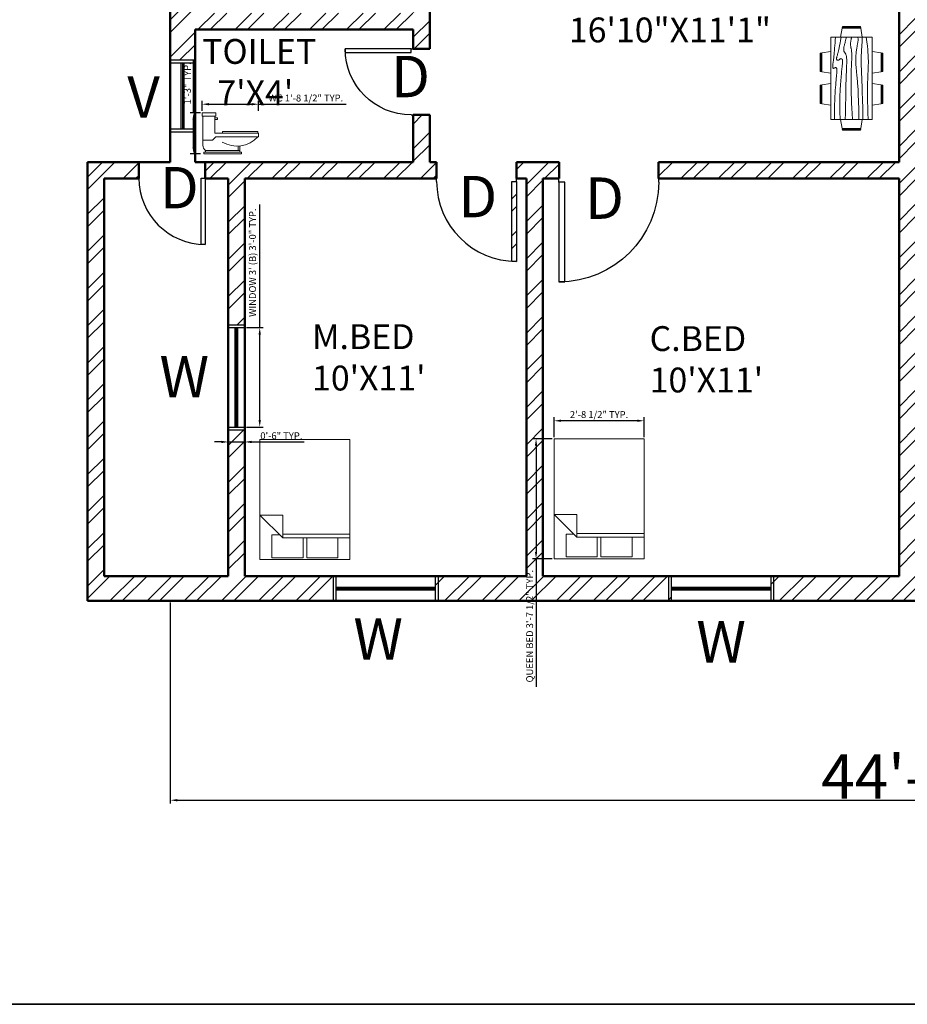
# Model space of a CAD drawing. Units: inches. Extents: x -31842 to -29388, y 18869 to 19743.
# Tile 5 of 12: x -30939 to -30617, y 18869 to 19226. Entities that reach past the tile are written whole.
import ezdxf

# ---------------------------------------------------------------- set-up
doc = ezdxf.new("R2010")
doc.units = ezdxf.units.IN
for name, color, linetype, lineweight in [('A-ANNO-DIMS', 2, 'Continuous', 18), ('A-ANNO-SYMB', 2, 'Continuous', 18), ('A-ANNO-TTLB', 7, 'Continuous', 35), ('A-AREA-IDEN', 3, 'Continuous', 18), ('A-DOOR', 3, 'Continuous', 25), ('A-FLOR-FIXT', 8, 'Continuous', 18), ('A-FURN', 8, 'Continuous', 18), ('A-GLAZ', 4, 'Continuous', 25), ('A-WALL', 7, 'Continuous', 50), ('A-WALL-PATT', 8, 'Continuous', 13)]:
    doc.layers.add(name, color=color, linetype=linetype, lineweight=lineweight)
doc.styles.get("Standard").update_dxf_attribs({"font": 'arial.ttf'})
doc.dimstyles.new('ISO-25', dxfattribs={"dimtxt": 2.5, "dimasz": 2.5, "dimexe": 1.25, "dimexo": 0.625, "dimtad": 1, "dimdec": 0, "dimlunit": 3, "dimtxsty": 'Standard', "dimcen": 2.5, "dimadec": 0, "dimazin": 0, "dimtfac": 1, "dimtdec": 0, "dimtmove": 0, "dimatfit": 3, "dimfxl": 1, "dimarcsym": 0})

# ---------------------------------------------------------------- blocks, each defined once
blk = doc.blocks.new('*U8')
for p, q in [((0, 0), (0, -100)), ((750, 0), (750, -100))]:
    blk.add_line(p, q)
blk.add_lwpolyline([(0, 0), (0, 750), (43.75, 750), (43.75, 0)], close=True)
blk.add_arc((0, 0), 750, 0, 90)
blk = doc.blocks.new('Bed - Queen')
for p, q in [((0, -80.00003), (0, 0)), ((0, 0), (59.99999, 0)), ((59.99999, 0), (59.99999, -80.00003)), ((7.99999, -1.2), (28.79998, -1.2)), ((7.99999, -14.4), (7.99999, -1.2)), ((28.79998, -1.2), (28.79998, -14.4)), ((31.19999, -1.2), (51.99999, -1.2)), ((31.19999, -14.4), (31.19999, -1.2)), ((51.99999, -1.2), (51.99999, -16.4)), ((0, -14.4), (44.8, -14.4)), ((44.8, -16.8), (0, -16.8)), ((59.99999, -29.6), (44.8, -14.4)), ((44.8, -14.4), (44.8, -29.6)), ((51.99999, -16.4), (46.79936, -16.4)), ((44.8, -29.6), (59.99999, -29.6)), ((59.99999, -80.00003), (0, -80.00003))]:
    blk.add_line(p, q)
blk = doc.blocks.new('Toilet - side')
for p, q in [((0.5, 5), (0.5, 22)), ((7.5, 22), (7.5, 12)), ((7.5, 21), (9, 21)), ((9, 20), (7.5, 20)), ((9, 21), (9, 20)), ((7.5, 12), (33, 12)), ((32.5, 13), (12, 13)), ((12, 13), (12, 12)), ((32.5, 12), (32.5, 13)), ((33, 12), (33, 10)), ((6, 8), (0.5, 8)), ((8, 10), (6, 8)), ((33, 10), (8, 10)), ((22, 2), (2, 2)), ((2, 2), (2, 1)), ((21, 4.5), (21, 2)), ((22, 2), (22, 4.54)), ((22, 1), (22, 2))]:
    blk.add_line(p, q)
for points in [[(0, 22), (0, 24), (8, 24), (8, 22)], [(1, 0), (1, 1), (23, 1), (23, 0)]]:
    blk.add_lwpolyline(points, close=True)
for centre, radius, start, end in [((20.3, 20.7), 16.23, 238.18715, 318.77023), ((3.75, 4.75), 3.26, 175.6013, 237.5288)]:
    blk.add_arc(centre, radius, start, end)
blk = doc.blocks.new('Dining Set - 36 x 72 in.')
for p, q in [((-22.2343, 26.00059), (-23.4847, 17.99762)), ((-22.2304, 26), (-5.7608, 26)), ((-22, 27.5), (-22.1562, 26.50042)), ((-5.8416, 26.5), (-22.1534, 26.5)), ((-22, 27.5), (-6, 27.5)), ((-5.8437, 26.49966), (-6, 27.5)), ((-4.5152, 17.99762), (-5.7655, 25.99926)), ((5.7657, 26.00059), (4.5153, 17.99762)), ((5.7696, 26), (22.2392, 26)), ((6, 27.5), (5.8438, 26.50042)), ((22.1584, 26.5), (5.8466, 26.5)), ((6, 27.5), (22, 27.5)), ((22.1563, 26.49966), (22, 27.5)), ((23.4848, 17.99762), (22.2345, 25.99926)), ((36, 18), (-36, 18)), ((-36, 18), (-36, -18)), ((36, -18), (36, 18)), ((-44.0006, 8.23428), (-35.9976, 9.48474)), ((44.0006, 8.23428), (35.9976, 9.48474)), ((-45.5, 8), (-44.5004, 8.15617)), ((-45.5, 8), (-45.5, -8)), ((-44.5, -8.15843), (-44.5, 8.15338)), ((-44, 8.23041), (-44, -8.23915)), ((44, 8.23041), (44, -8.23915)), ((44.5, -8.15843), (44.5, 8.15338)), ((45.5, 8), (44.5005, 8.15617)), ((45.5, 8), (45.5, -8)), ((-44.4997, -8.15631), (-45.5, -8)), ((-35.9976, -9.48476), (-43.9993, -8.2345)), ((35.9976, -9.48476), (43.9993, -8.2345)), ((44.4997, -8.15631), (45.5, -8)), ((-36, -18), (36, -18)), ((-22.2343, -26.0006), (-23.4847, -17.99762)), ((-4.5152, -17.99762), (-5.7655, -25.99928)), ((5.7657, -26.0006), (4.5153, -17.99762)), ((23.4848, -17.99762), (22.2345, -25.99928)), ((-22.2304, -26), (-5.7608, -26)), ((-22, -27.5), (-22.1562, -26.50044)), ((-5.8416, -26.5), (-22.1534, -26.5)), ((-22, -27.5), (-6, -27.5)), ((-5.8437, -26.49967), (-6, -27.5)), ((5.7696, -26), (22.2392, -26)), ((6, -27.5), (5.8438, -26.50044)), ((22.1584, -26.5), (5.8466, -26.5)), ((6, -27.5), (22, -27.5)), ((22.1563, -26.49967), (22, -27.5))]:
    blk.add_line(p, q)
for points in [[(-36, 15), (-31.1772, 14.97754), (-26.8079, 14.91406), (-22.8538, 14.81543), (-19.276, 14.6875), (-16.0362, 14.53613), (-13.0957, 14.36718), (-10.4159, 14.18652), (-7.9583, 14), (-5.6904, 13.81315), (-3.6035, 13.63021), (-1.6954, 13.45508), (0.0365, 13.29166), (1.5945, 13.14388), (2.9811, 13.01562), (4.1988, 12.9108), (5.25, 12.83333), (6.1393, 12.78613), (6.8802, 12.76823), (7.4883, 12.77767), (7.9792, 12.8125), (8.3685, 12.87077), (8.6719, 12.95052), (8.9049, 13.0498), (9.0833, 13.16666), (9.2205, 13.29899), (9.3216, 13.44401), (9.3895, 13.59879), (9.4271, 13.76041), (9.4373, 13.92594), (9.4232, 14.09245), (9.3875, 14.257), (9.3333, 14.41666), (9.2638, 14.56917), (9.1836, 14.71484), (9.0975, 14.85465), (9.0104, 14.98958), (8.9272, 15.1206), (8.8529, 15.2487), (8.7922, 15.37483), (8.75, 15.5), (8.7305, 15.62467), (8.7344, 15.74739), (8.7617, 15.86621), (8.8125, 15.97916), (8.8867, 16.08431), (8.9844, 16.17968), (9.1055, 16.26334), (9.25, 16.33333), (9.4189, 16.38802), (9.6172, 16.42708), (9.8506, 16.45052), (10.125, 16.45833), (10.4463, 16.45052), (10.8203, 16.42708), (11.2529, 16.38802), (11.75, 16.33333), (12.3184, 16.26318), (12.9694, 16.17838), (13.7151, 16.07991), (14.5677, 15.96875), (15.5395, 15.84586), (16.6426, 15.71224), (17.8893, 15.56884), (19.2917, 15.41666), (20.859, 15.25667), (22.5879, 15.08984), (24.4721, 14.91715), (26.5052, 14.73958), (28.6809, 14.5581), (30.9929, 14.3737), (33.4347, 14.18733), (36, 14)], [(-36, 10), (-28.9766, 10.14274), (-23.1725, 10.20442), (-18.4241, 10.19775), (-14.5677, 10.13541), (-11.4399, 10.03011), (-8.877, 9.89453), (-6.7154, 9.74137), (-4.7917, 9.58333), (-2.9698, 9.43082), (-1.2246, 9.28515), (0.4415, 9.14534), (2.026, 9.01041), (3.5266, 8.87939), (4.9408, 8.7513), (6.266, 8.62516), (7.5, 8.5), (8.6411, 8.37549), (9.6914, 8.2539), (10.6538, 8.13818), (11.5312, 8.03125), (12.3267, 7.93603), (13.043, 7.85547), (13.6831, 7.79248), (14.25, 7.75), (14.7471, 7.7303), (15.1797, 7.73307), (15.5537, 7.75732), (15.875, 7.80208), (16.1494, 7.86637), (16.3828, 7.94922), (16.5811, 8.04964), (16.75, 8.16666), (16.8944, 8.29915), (17.0143, 8.44531), (17.1089, 8.60319), (17.1771, 8.77083), (17.218, 8.94629), (17.2305, 9.1276), (17.2137, 9.31282), (17.1667, 9.5), (17.0895, 9.6875), (16.987, 9.875), (16.8649, 10.0625), (16.7292, 10.25), (16.5856, 10.4375), (16.4401, 10.625), (16.2985, 10.8125), (16.1667, 11), (16.05, 11.18733), (15.9518, 11.3737), (15.8752, 11.5581), (15.8229, 11.73958), (15.798, 11.91715), (15.8034, 12.08984), (15.842, 12.25667), (15.9167, 12.41666), (16.0295, 12.56836), (16.1784, 12.70833), (16.3605, 12.83268), (16.5729, 12.9375), (16.8127, 13.01888), (17.0768, 13.07291), (17.3625, 13.0957), (17.6667, 13.08333), (17.9894, 13.03312), (18.3418, 12.94726), (18.7382, 12.82918), (19.1927, 12.68229), (19.7195, 12.51001), (20.3327, 12.31575), (21.0465, 12.10294), (21.875, 11.875), (22.8357, 11.63354), (23.959, 11.37304), (25.2786, 11.08618), (26.8282, 10.76562), (28.6414, 10.40405), (30.752, 9.99414), (33.1936, 9.52856), (36, 9)], [(-36, 5.5), (-30.7157, 5.3348), (-26.069, 5.20963), (-21.9946, 5.11767), (-18.4271, 5.05208), (-15.3009, 5.00602), (-12.5508, 4.97265), (-10.1112, 4.94515), (-7.9167, 4.91666), (-5.909, 4.88167), (-4.0586, 4.83984), (-2.3429, 4.79215), (-0.7396, 4.73958), (0.7739, 4.6831), (2.22, 4.6237), (3.6213, 4.56233), (5, 4.5), (6.373, 4.43782), (7.7344, 4.3776), (9.0723, 4.32129), (10.375, 4.27083), (11.6309, 4.22819), (12.8281, 4.19531), (13.9551, 4.17415), (15, 4.16666), (15.954, 4.17448), (16.819, 4.19791), (17.6001, 4.23698), (18.3021, 4.29166), (18.9299, 4.36198), (19.4883, 4.44791), (19.9823, 4.54948), (20.4167, 4.66666), (20.7969, 4.79899), (21.1302, 4.94401), (21.4245, 5.09879), (21.6875, 5.26041), (21.9271, 5.42594), (22.1511, 5.59245), (22.3672, 5.757), (22.5834, 5.91666), (22.8065, 6.06868), (23.0404, 6.21093), (23.2879, 6.34147), (23.5521, 6.45833), (23.8358, 6.55957), (24.142, 6.64323), (24.4735, 6.70735), (24.8334, 6.75), (25.2235, 6.76969), (25.642, 6.76692), (26.0858, 6.74267), (26.5521, 6.69791), (27.0379, 6.63362), (27.5404, 6.55078), (28.0565, 6.45036), (28.5834, 6.33333), (29.1242, 6.19987), (29.7071, 6.04687), (30.3661, 5.87044), (31.1354, 5.66666), (32.0493, 5.43164), (33.142, 5.16146), (34.4475, 4.85221), (36, 4.5)], [(-36, -1), (-30.7915, -0.6591), (-26.0195, -0.38216), (-21.6519, -0.16284), (-17.6563, 0.00521), (-14.0005, 0.12833), (-10.6523, 0.21289), (-7.5796, 0.26522), (-4.75, 0.29166), (-2.134, 0.29793), (0.2878, 0.28711), (2.5317, 0.26163), (4.6146, 0.22396), (6.5529, 0.17651), (8.3633, 0.12174), (10.0623, 0.06209), (11.6667, 0), (13.1899, -0.06201), (14.6341, -0.1211), (15.9982, -0.17432), (17.2813, -0.21875), (18.4823, -0.25147), (19.6003, -0.26953), (20.6343, -0.27002), (21.5834, -0.25), (22.4481, -0.20768), (23.2357, -0.14584), (23.9549, -0.06836), (24.6146, 0.02083), (25.2235, 0.11784), (25.7904, 0.21875), (26.3241, 0.31966), (26.8334, 0.41666), (27.3265, 0.50618), (27.8099, 0.58593), (28.2894, 0.65397), (28.7709, 0.70833), (29.2601, 0.74707), (29.763, 0.76823), (30.2855, 0.76985), (30.8334, 0.75), (31.4088, 0.70784), (31.9994, 0.64713), (32.589, 0.57275), (33.1615, 0.48958), (33.7008, 0.4025), (34.1908, 0.3164), (34.6153, 0.23616), (34.9584, 0.16666), (35.2099, 0.11165), (35.3848, 0.07031), (35.504, 0.04069), (35.5886, 0.02083), (35.6594, 0.00879), (35.7377, 0.0026), (35.8442, 0.00032), (36, 0)], [(-36, -6.5), (-27.1843, -6.31267), (-20.084, -6.1263), (-14.469, -5.9419), (-10.1094, -5.76042), (-6.7752, -5.58285), (-4.2363, -5.41016), (-2.2629, -5.24333), (-0.625, -5.08334), (0.8708, -4.93099), (2.2715, -4.78646), (3.5872, -4.64974), (4.8281, -4.52084), (6.0046, -4.39974), (7.127, -4.28646), (8.2053, -4.18099), (9.25, -4.08334), (10.2705, -3.99382), (11.2734, -3.91407), (12.2647, -3.84603), (13.25, -3.79167), (14.2354, -3.75293), (15.2266, -3.73177), (16.2295, -3.73015), (17.25, -3.75), (18.2912, -3.79248), (19.3451, -3.85547), (20.4009, -3.93604), (21.4479, -4.03125), (22.4754, -4.13819), (23.4727, -4.25391), (24.4289, -4.37549), (25.3334, -4.5), (26.1785, -4.62492), (26.9694, -4.74935), (27.7145, -4.87281), (28.4219, -4.99479), (29.1, -5.11483), (29.7572, -5.23242), (30.4016, -5.34709), (31.0417, -5.45834), (31.6837, -5.56437), (32.3262, -5.65821), (32.9658, -5.73153), (33.599, -5.77604), (34.2224, -5.78345), (34.8327, -5.74545), (35.4264, -5.65373), (36, -5.5)], [(-36, -10), (-26.4022, -9.81299), (-18.4675, -9.62891), (-11.9839, -9.45069), (-6.7396, -9.28125), (-2.5226, -9.12354), (0.8789, -8.98047), (3.6769, -8.85498), (6.0833, -8.75), (8.2767, -8.66765), (10.3021, -8.60677), (12.1712, -8.56543), (13.8958, -8.54167), (15.4876, -8.53353), (16.9583, -8.53907), (18.3197, -8.55632), (19.5834, -8.58334), (20.7616, -8.61841), (21.8685, -8.66081), (22.9188, -8.71004), (23.9271, -8.76563), (24.9081, -8.82707), (25.8763, -8.89388), (26.8465, -8.96558), (27.8334, -9.04167), (28.8474, -9.12118), (29.8828, -9.20117), (30.93, -9.27824), (31.9792, -9.34896), (33.0205, -9.40991), (34.0443, -9.45768), (35.0407, -9.48885), (36, -9.5)], [(-36, -14.5), (-30.0881, -14.33513), (-25.0332, -14.21224), (-20.7312, -14.12647), (-17.0781, -14.07292), (-13.97, -14.04671), (-11.3027, -14.04297), (-8.9724, -14.05681), (-6.875, -14.08334), (-4.9224, -14.11833), (-3.0905, -14.16016), (-1.3709, -14.20785), (0.2448, -14.26042), (1.7647, -14.3169), (3.1973, -14.3763), (4.5507, -14.43767), (5.8333, -14.5), (7.0554, -14.5621), (8.235, -14.62175), (9.3922, -14.67652), (10.5469, -14.72396), (11.7192, -14.76164), (12.929, -14.78711), (14.1965, -14.79794), (15.5417, -14.79167), (16.9933, -14.76424), (18.6152, -14.70508), (20.4804, -14.60197), (22.6615, -14.44271), (25.2312, -14.21509), (28.2624, -13.9069), (31.8277, -13.50594), (36, -13)]]:
    blk.add_lwpolyline(points)
blk = doc.blocks.new('*D204')
at = {"layer": 'A-ANNO-DIMS', "color": 0, "lineweight": -2, "transparency": 16777216}
for p, q in [((-30884.39, 19014.34), (-30884.39, 18941.51)), ((-30352.39, 19014.34), (-30352.39, 18941.51)), ((-30881.89, 18942.76), (-30354.89, 18942.76))]:
    blk.add_line(p, q, dxfattribs=at)
at = {"layer": 'A-ANNO-DIMS', "color": 0, "transparency": 16777216}
for points in [[(-30881.89, 18943.17), (-30881.89, 18942.34), (-30884.39, 18942.76)], [(-30354.89, 18943.17), (-30354.89, 18942.34), (-30352.39, 18942.76)]]:
    blk.add_solid(points, dxfattribs=at)
at = {"layer": 'Defpoints', "color": 0, "transparency": 16777216}
for p in [(-30884.39, 19014.96), (-30352.39, 19014.96), (-30352.39, 18942.76)]:
    blk.add_point(p, dxfattribs=at)
at = {"layer": 'A-ANNO-DIMS', "color": 0, "transparency": 16777216, "insert": (-30618.39, 18951.38), "char_height": 2.5, "attachment_point": 5}
blk.add_mtext('{\\H6.4x;44\'-4"}', dxfattribs=at)
blk = doc.blocks.new('WIN-3FT')
for p, q in [((0, 36), (9, 36)), ((4, 0), (4, 36)), ((4.5, 0), (4.5, 36)), ((5, 0), (5, 36)), ((0, 0), (9, 0))]:
    blk.add_line(p, q)
blk = doc.blocks.new('WIN-3FT-B')
for p, q in [((0, 36), (6, 36)), ((2.5, 0), (2.5, 36)), ((3, 0), (3, 36)), ((3.5, 0), (3.5, 36)), ((0, 0), (6, 0))]:
    blk.add_line(p, q)
blk = doc.blocks.new('WIN-2FT')
for p, q in [((0, 24), (9, 24)), ((4, 0), (4, 24)), ((4.5, 0), (4.5, 24)), ((5, 0), (5, 24)), ((0, 0), (9, 0))]:
    blk.add_line(p, q)
blk = doc.blocks.new('*D221')
at = {"layer": 'A-ANNO-DIMS', "color": 0, "lineweight": -2, "transparency": 16777216}
for p, q in [((-30745.99, 19073.71), (-30753.13, 19073.71)), ((-30751.88, 19071.21), (-30751.88, 19032.73)), ((-30745.99, 19030.23), (-30753.13, 19030.23)), ((-30751.88, 19030.23), (-30751.88, 18983.88))]:
    blk.add_line(p, q, dxfattribs=at)
at = {"layer": 'A-ANNO-DIMS', "color": 0, "transparency": 16777216}
for points in [[(-30752.3, 19071.21), (-30751.47, 19071.21), (-30751.88, 19073.71)], [(-30752.3, 19032.73), (-30751.47, 19032.73), (-30751.88, 19030.23)]]:
    blk.add_solid(points, dxfattribs=at)
at = {"layer": 'Defpoints', "color": 0, "transparency": 16777216}
for p in [(-30745.36, 19073.71), (-30751.88, 19030.23), (-30745.36, 19030.23)]:
    blk.add_point(p, dxfattribs=at)
at = {"layer": 'A-ANNO-DIMS', "color": 0, "transparency": 16777216, "insert": (-30753.88, 19005.8), "char_height": 2.5, "attachment_point": 5, "rotation": 90}
blk.add_mtext('QUEEN BED 3\'-7 1/2" TYP.', dxfattribs=at)
blk = doc.blocks.new('*D222')
at = {"layer": 'A-ANNO-DIMS', "color": 0, "lineweight": -2, "transparency": 16777216}
for p, q in [((-30745.36, 19074.34), (-30745.36, 19081.48)), ((-30712.75, 19074.34), (-30712.75, 19081.48)), ((-30715.25, 19080.23), (-30742.86, 19080.23))]:
    blk.add_line(p, q, dxfattribs=at)
at = {"layer": 'A-ANNO-DIMS', "color": 0, "transparency": 16777216}
for points in [[(-30742.86, 19080.65), (-30742.86, 19079.82), (-30745.36, 19080.23)], [(-30715.25, 19080.65), (-30715.25, 19079.82), (-30712.75, 19080.23)]]:
    blk.add_solid(points, dxfattribs=at)
at = {"layer": 'Defpoints', "color": 0, "transparency": 16777216}
for p in [(-30745.36, 19080.23), (-30745.36, 19073.71), (-30712.75, 19073.71)]:
    blk.add_point(p, dxfattribs=at)
at = {"layer": 'A-ANNO-DIMS', "color": 0, "transparency": 16777216, "insert": (-30729.06, 19082.15), "char_height": 2.5, "attachment_point": 5}
blk.add_mtext('2\'-8 1/2" TYP.', dxfattribs=at)
blk = doc.blocks.new('*D227')
at = {"layer": 'A-ANNO-DIMS', "color": 0, "lineweight": -2, "transparency": 16777216}
for p, q in [((-30872.87, 19192.46), (-30872.87, 19196.16)), ((-30870.37, 19194.91), (-30854.88, 19194.91)), ((-30852.38, 19192.46), (-30852.38, 19196.16)), ((-30852.38, 19194.91), (-30820.67, 19194.91))]:
    blk.add_line(p, q, dxfattribs=at)
at = {"layer": 'A-ANNO-DIMS', "color": 0, "transparency": 16777216}
for points in [[(-30870.37, 19195.33), (-30870.37, 19194.5), (-30872.87, 19194.91)], [(-30854.88, 19195.33), (-30854.88, 19194.5), (-30852.38, 19194.91)]]:
    blk.add_solid(points, dxfattribs=at)
at = {"layer": 'Defpoints', "color": 0, "transparency": 16777216}
for p in [(-30852.38, 19194.91), (-30872.87, 19191.84), (-30852.38, 19191.84)]:
    blk.add_point(p, dxfattribs=at)
at = {"layer": 'A-ANNO-DIMS', "color": 0, "transparency": 16777216, "insert": (-30835.28, 19196.83), "char_height": 2.5, "attachment_point": 5}
blk.add_mtext('WC 1\'-8 1/2" TYP.', dxfattribs=at)
blk = doc.blocks.new('*D228')
at = {"layer": 'A-ANNO-DIMS', "color": 0, "lineweight": -2, "transparency": 16777216}
for p, q in [((-30875.95, 19191.84), (-30875.95, 19210.59)), ((-30873.5, 19191.84), (-30877.2, 19191.84)), ((-30875.95, 19179.43), (-30875.95, 19189.34)), ((-30873.5, 19176.93), (-30877.2, 19176.93))]:
    blk.add_line(p, q, dxfattribs=at)
at = {"layer": 'A-ANNO-DIMS', "color": 0, "transparency": 16777216}
for points in [[(-30876.36, 19189.34), (-30875.53, 19189.34), (-30875.95, 19191.84)], [(-30876.36, 19179.43), (-30875.53, 19179.43), (-30875.95, 19176.93)]]:
    blk.add_solid(points, dxfattribs=at)
at = {"layer": 'Defpoints', "color": 0, "transparency": 16777216}
for p in [(-30875.95, 19191.84), (-30872.87, 19191.84), (-30872.87, 19176.93)]:
    blk.add_point(p, dxfattribs=at)
at = {"layer": 'A-ANNO-DIMS', "color": 0, "transparency": 16777216, "insert": (-30877.85, 19202.47), "char_height": 2.5, "attachment_point": 5, "rotation": 90}
blk.add_mtext('1\'-3" TYP.', dxfattribs=at)
blk = doc.blocks.new('*D257')
at = {"layer": 'A-ANNO-DIMS', "color": 0, "lineweight": -2, "transparency": 16777216}
for p, q in [((-30851.99, 19113.96), (-30851.99, 19158.55)), ((-30856.77, 19113.96), (-30850.74, 19113.96)), ((-30851.99, 19080.46), (-30851.99, 19111.46)), ((-30856.77, 19077.96), (-30850.74, 19077.96))]:
    blk.add_line(p, q, dxfattribs=at)
at = {"layer": 'A-ANNO-DIMS', "color": 0, "transparency": 16777216}
for points in [[(-30852.41, 19111.46), (-30851.58, 19111.46), (-30851.99, 19113.96)], [(-30852.41, 19080.46), (-30851.58, 19080.46), (-30851.99, 19077.96)]]:
    blk.add_solid(points, dxfattribs=at)
at = {"layer": 'Defpoints', "color": 0, "transparency": 16777216}
for p in [(-30857.39, 19113.96), (-30851.99, 19113.96), (-30857.39, 19077.96)]:
    blk.add_point(p, dxfattribs=at)
at = {"layer": 'A-ANNO-DIMS', "color": 0, "transparency": 16777216, "insert": (-30854.26, 19137.51), "char_height": 2.5, "attachment_point": 5, "rotation": 90}
blk.add_mtext('WINDOW 3\' (B) 3\'-0" TYP.', dxfattribs=at)
blk = doc.blocks.new('*D258')
at = {"layer": 'A-ANNO-DIMS', "color": 0, "lineweight": -2, "transparency": 16777216}
for p, q in [((-30863.39, 19077.34), (-30863.39, 19071.31)), ((-30857.39, 19077.34), (-30857.39, 19071.31)), ((-30865.89, 19072.56), (-30868.39, 19072.56)), ((-30863.39, 19072.56), (-30857.39, 19072.56)), ((-30854.89, 19072.56), (-30835.9, 19072.56))]:
    blk.add_line(p, q, dxfattribs=at)
at = {"layer": 'A-ANNO-DIMS', "color": 0, "transparency": 16777216}
for points in [[(-30865.89, 19072.98), (-30865.89, 19072.14), (-30863.39, 19072.56)], [(-30854.89, 19072.98), (-30854.89, 19072.14), (-30857.39, 19072.56)]]:
    blk.add_solid(points, dxfattribs=at)
at = {"layer": 'Defpoints', "color": 0, "transparency": 16777216}
for p in [(-30863.39, 19077.96), (-30857.39, 19077.96), (-30857.39, 19072.56)]:
    blk.add_point(p, dxfattribs=at)
at = {"layer": 'A-ANNO-DIMS', "color": 0, "transparency": 16777216, "insert": (-30844.15, 19074.46), "char_height": 2.5, "attachment_point": 5}
blk.add_mtext('0\'-6" TYP.', dxfattribs=at)

msp = doc.modelspace()

# ---------------------------------------------------------------- hatches: boundary and pattern name
at = {"layer": 'A-WALL-PATT'}
h = msp.add_hatch(dxfattribs=at)
h.set_pattern_fill('ANSI32', color=256)
h.paths.add_polyline_path([(-30352.39, 19656.96), (-30487.39, 19656.96), (-30487.39, 19614.96), (-30510.39, 19614.96), (-30510.39, 19605.96), (-30487.39, 19605.96), (-30487.39, 19558.38), (-30481.39, 19558.38), (-30481.39, 19605.96), (-30469.68, 19605.96), (-30469.68, 19614.96), (-30481.39, 19614.96), (-30481.39, 19650.96), (-30361.39, 19650.96), (-30361.39, 19614.96), (-30445.68, 19614.96), (-30445.68, 19605.96), (-30361.39, 19605.96), (-30361.39, 19564.96), (-30352.39, 19564.96)])
h.paths.add_polyline_path([(-30548.39, 19614.96), (-30599.39, 19614.96), (-30599.39, 19605.96), (-30577.39, 19605.96), (-30577.39, 19457.87), (-30571.39, 19457.87), (-30571.39, 19491.96), (-30560.76, 19491.96), (-30560.76, 19497.96), (-30571.39, 19497.96), (-30571.39, 19605.96), (-30548.39, 19605.96)])
h.paths.add_polyline_path([(-30637.39, 19614.96), (-30688.39, 19614.96), (-30688.39, 19605.96), (-30665.39, 19605.96), (-30665.39, 19497.96), (-30682.48, 19497.96), (-30682.48, 19491.96), (-30665.39, 19491.96), (-30665.39, 19454.79), (-30662.43, 19454.79), (-30659.39, 19454.79), (-30659.39, 19605.96), (-30637.39, 19605.96)])
h.paths.add_polyline_path([(-30789.63, 19614.96), (-30875.39, 19614.96), (-30875.39, 19650.96), (-30755.39, 19650.96), (-30755.39, 19614.96), (-30765.63, 19614.96), (-30765.63, 19605.96), (-30755.39, 19605.96), (-30755.39, 19550.68), (-30749.39, 19550.68), (-30749.39, 19605.96), (-30726.39, 19605.96), (-30726.39, 19614.96), (-30749.39, 19614.96), (-30749.39, 19656.96), (-30884.39, 19656.96), (-30884.39, 19564.96), (-30875.39, 19564.96), (-30875.39, 19605.96), (-30789.63, 19605.96)])
h.paths.add_polyline_path([(-30749.39, 19491.96), (-30736.92, 19491.96), (-30736.92, 19494.96), (-30682.48, 19494.96), (-30682.48, 19497.96), (-30665.39, 19497.96), (-30665.39, 19605.96), (-30688.39, 19605.96), (-30749.39, 19605.96), (-30749.39, 19550.68), (-30755.39, 19550.68), (-30757.34, 19550.71, 0.39722), (-30793.34, 19516.76), (-30757.34, 19516.76), (-30757.34, 19514.65), (-30793.4, 19514.65), (-30793.4, 19516.76), (-30793.34, 19516.76, -0.39722), (-30757.34, 19550.71), (-30755.39, 19550.71), (-30755.39, 19605.96), (-30765.63, 19605.96), (-30765.63, 19613.66), (-30767.03, 19613.66), (-30767.03, 19637.62, 0.397344), (-30789.63, 19613.65), (-30789.63, 19605.96), (-30875.39, 19605.96), (-30875.39, 19564.96), (-30875.39, 19485.96), (-30873.79, 19485.96), (-30873.79, 19479.96), (-30873.79, 19479.35, 0.39722), (-30851.19, 19455.39), (-30851.19, 19479.35), (-30849.79, 19479.35), (-30849.79, 19455.34), (-30851.19, 19455.34), (-30851.19, 19455.39, -0.39722), (-30873.79, 19479.35), (-30873.79, 19479.96), (-30875.39, 19479.96), (-30875.39, 19431.96), (-30848.39, 19431.96), (-30848.39, 19468.96), (-30842.39, 19468.96), (-30842.39, 19479.96), (-30755.39, 19479.96), (-30755.39, 19470.97), (-30749.39, 19470.97)])
h.paths.add_polyline_path([(-30738.39, 19585.51), (-30738.39, 19586.08), (-30736.12, 19586.08), (-30736.12, 19586.65), (-30739.53, 19586.65), (-30739.53, 19600.27), (-30722.5, 19600.27), (-30722.5, 19586.65), (-30725.91, 19586.65), (-30725.91, 19586.08), (-30723.64, 19586.08), (-30723.64, 19585.51)], flags=16)
h.paths.add_polyline_path([(-30737.83, 19590.05, -1), (-30734.42, 19590.05, -1)], flags=16)
h.paths.add_polyline_path([(-30737.26, 19590.05, -1), (-30734.99, 19590.05, -1)], flags=0)
h.paths.add_polyline_path([(-30732.72, 19588.35), (-30732.72, 19597.43), (-30729.31, 19597.43), (-30729.31, 19588.35)], flags=16)
h.paths.add_polyline_path([(-30736.69, 19590.05, -1), (-30735.56, 19590.05, -1)], flags=0)
h.paths.add_polyline_path([(-30732.15, 19588.92), (-30732.15, 19596.86), (-30729.88, 19596.86), (-30729.88, 19588.92)], flags=0)
h.paths.add_polyline_path([(-30728.18, 19590.05, -1), (-30723.64, 19590.05, -1)], flags=0)
h.paths.add_polyline_path([(-30727.61, 19590.05, -1), (-30724.2, 19590.05, -1)], flags=0)
h.paths.add_polyline_path([(-30727.04, 19590.05, -1), (-30724.77, 19590.05, -1)], flags=0)
h.paths.add_polyline_path([(-30726.47, 19590.05, -1), (-30725.34, 19590.05, -1)], flags=0)
h.paths.add_polyline_path([(-30738.39, 19595.16, -1), (-30733.85, 19595.16, -1)], flags=16)
h.paths.add_polyline_path([(-30737.83, 19595.16, -1), (-30734.42, 19595.16, -1)], flags=0)
h.paths.add_polyline_path([(-30737.26, 19595.16, -1), (-30734.99, 19595.16, -1)], flags=0)
h.paths.add_polyline_path([(-30736.69, 19595.16, -1), (-30735.56, 19595.16, -1)], flags=0)
h.paths.add_polyline_path([(-30727.61, 19595.16, -1), (-30724.2, 19595.16, -1)], flags=0)
h.paths.add_polyline_path([(-30727.04, 19595.16, -1), (-30724.77, 19595.16, -1)], flags=0)
h.paths.add_polyline_path([(-30707.55, 19587.34, -0.414214), (-30708.36, 19588.14), (-30708.36, 19597.29, -0.414214), (-30707.55, 19598.09), (-30693.03, 19598.09, -0.414214), (-30692.23, 19597.29), (-30692.23, 19588.14, -0.414214), (-30693.03, 19587.34)], flags=16)
h.paths.add_polyline_path([(-30726.47, 19595.16, -1), (-30725.34, 19595.16, -1)], flags=0)
h.paths.add_polyline_path([(-30827.74, 19570.11), (-30871.22, 19570.11), (-30871.22, 19602.72), (-30827.74, 19602.72)], flags=16)
h.paths.add_polyline_path([(-30707.01, 19588.14, -0.414214), (-30707.55, 19588.68), (-30707.55, 19594.6, -0.414214), (-30707.01, 19595.13), (-30693.57, 19595.13, -0.414214), (-30693.03, 19594.6), (-30693.03, 19588.68, -0.414214), (-30693.57, 19588.14)], flags=0)
h.paths.add_polyline_path([(-30700.02, 19591.64, -1), (-30700.56, 19591.64, -1)], flags=0)
h.paths.add_polyline_path([(-30863.39, 19594.46), (-30863.39, 19574.46), (-30870.57, 19574.46), (-30870.57, 19585.76), (-30863.39, 19585.76), (-30863.39, 19587.07), (-30870.57, 19587.07), (-30870.57, 19598.37), (-30862.31, 19598.37), (-30862.31, 19595.55), (-30855.13, 19602.72), (-30855.13, 19594.46)], flags=0)
h.paths.add_polyline_path([(-30755.39, 19514.65), (-30757.34, 19514.65), (-30793.4, 19514.65), (-30793.4, 19516.76), (-30793.34, 19516.76, -0.39722), (-30757.34, 19550.71), (-30755.39, 19550.71), (-30755.39, 19605.96), (-30765.63, 19605.96), (-30765.63, 19613.66), (-30767.03, 19613.66), (-30767.03, 19637.62, 0.397344), (-30789.63, 19613.65), (-30789.63, 19605.96), (-30875.39, 19605.96), (-30875.39, 19564.96), (-30875.39, 19485.96), (-30873.79, 19485.96), (-30873.79, 19479.96), (-30873.79, 19479.35, 0.39722), (-30851.19, 19455.39), (-30851.19, 19479.35), (-30849.79, 19479.35), (-30849.79, 19479.96), (-30849.79, 19479.96), (-30849.79, 19485.96), (-30755.39, 19485.96)], flags=16)
h.paths.add_polyline_path([(-30665.39, 19605.96), (-30688.39, 19605.96), (-30749.39, 19605.96), (-30749.39, 19550.68), (-30755.39, 19550.68), (-30757.34, 19550.71, 0.39722), (-30793.34, 19516.76), (-30757.34, 19516.76), (-30757.34, 19514.65), (-30755.39, 19514.65), (-30755.39, 19514.68), (-30749.39, 19514.68), (-30749.39, 19497.96), (-30736.92, 19497.96), (-30736.92, 19494.96), (-30682.48, 19494.96), (-30682.48, 19497.96), (-30665.39, 19497.96)], flags=17)
h.paths.add_polyline_path([(-30749.39, 19446.97), (-30755.39, 19446.97), (-30755.39, 19431.96), (-30842.39, 19431.96), (-30842.39, 19442.96), (-30848.39, 19442.96), (-30848.39, 19431.96), (-30875.39, 19431.96), (-30875.39, 19479.96), (-30873.79, 19479.96), (-30873.79, 19482.55), (-30873.79, 19485.96), (-30875.39, 19485.96), (-30875.39, 19526.96), (-30884.39, 19526.96), (-30884.39, 19384.96), (-30875.39, 19384.96), (-30875.39, 19425.96), (-30755.39, 19425.96), (-30755.39, 19414.67), (-30751.3, 19414.67), (-30749.39, 19414.62)])
h.paths.add_polyline_path([(-30848.39, 19468.96), (-30848.39, 19479.96), (-30849.79, 19479.96), (-30849.79, 19479.35), (-30849.79, 19455.34), (-30851.19, 19455.34), (-30851.19, 19455.39, -0.39722), (-30873.79, 19479.35), (-30873.79, 19479.96), (-30875.39, 19479.96), (-30875.39, 19431.96), (-30848.39, 19431.96), (-30848.39, 19442.96)], flags=17)
h.paths.add_polyline_path([(-30659.39, 19407.96), (-30657.22, 19407.96), (-30657.22, 19413.96), (-30659.39, 19413.96), (-30659.39, 19418.79), (-30665.39, 19418.79), (-30665.39, 19305.96), (-30749.39, 19305.96), (-30749.39, 19378.62), (-30755.39, 19378.62), (-30755.39, 19305.96), (-30875.39, 19305.96), (-30875.39, 19346.96), (-30884.39, 19346.96), (-30884.39, 19282.96), (-30875.39, 19282.96), (-30875.39, 19299.96), (-30796.39, 19299.96), (-30796.39, 19286.68), (-30790.39, 19286.68), (-30790.39, 19299.96), (-30659.39, 19299.96)])
h.paths.add_polyline_path([(-30352.39, 19346.96), (-30361.39, 19346.96), (-30361.39, 19305.96), (-30481.39, 19305.96), (-30481.39, 19380.1), (-30487.39, 19380.1), (-30487.39, 19305.96), (-30571.39, 19305.96), (-30571.39, 19421.87), (-30577.39, 19421.87), (-30577.39, 19413.96), (-30579.53, 19413.96), (-30579.53, 19407.96), (-30577.39, 19407.96), (-30577.39, 19299.96), (-30446.39, 19299.96), (-30446.39, 19291.76), (-30440.39, 19291.76), (-30440.39, 19299.96), (-30361.39, 19299.96), (-30361.39, 19282.96), (-30352.39, 19282.96)])
h.paths.add_polyline_path([(-30481.39, 19449.62), (-30484.39, 19449.62), (-30487.39, 19449.62), (-30487.39, 19416.1), (-30481.39, 19416.1), (-30481.39, 19425.96), (-30361.39, 19425.96), (-30361.39, 19384.96), (-30352.39, 19384.96), (-30352.39, 19526.96), (-30361.39, 19526.96), (-30361.39, 19485.96), (-30363.32, 19485.96), (-30363.32, 19479.96), (-30361.39, 19479.96), (-30361.39, 19431.96), (-30388.39, 19431.96), (-30388.39, 19442.96), (-30394.39, 19442.96), (-30394.39, 19431.96), (-30481.39, 19431.96)])
h.paths.add_polyline_path([(-30387.32, 19482.76), (-30387.32, 19485.96), (-30481.39, 19485.96), (-30481.39, 19522.38), (-30487.39, 19522.38), (-30487.39, 19497.96), (-30500.08, 19497.96), (-30500.08, 19491.96), (-30487.39, 19491.96), (-30487.39, 19473.62), (-30481.39, 19473.62), (-30481.39, 19479.96), (-30394.39, 19479.96), (-30394.39, 19468.96), (-30388.39, 19468.96), (-30388.39, 19479.96), (-30387.32, 19479.96)])
h.paths.add_polyline_path([(-30626.04, 19413.96), (-30610.58, 19413.96), (-30610.58, 19407.24), (-30608.81, 19407.24), (-30608.81, 19376.14), (-30610.63, 19376.14), (-30610.63, 19407.96), (-30614.39, 19407.96), (-30614.39, 19173.96), (-30532.79, 19173.96), (-30532.79, 19167.96), (-30532.79, 19166.59), (-30532.79, 19167.96), (-30614.39, 19167.96), (-30614.39, 19023.96), (-30568.89, 19023.96), (-30568.89, 19014.96), (-30666.89, 19014.96), (-30666.89, 19018.96), (-30702.89, 19018.96), (-30702.89, 19019.96), (-30666.89, 19019.96), (-30666.89, 19023.96), (-30620.39, 19023.96), (-30620.39, 19167.96), (-30707.45, 19167.96), (-30707.45, 19166.65, -0.39722), (-30741.49, 19130.57), (-30741.49, 19130.51), (-30743.6, 19130.51), (-30743.6, 19166.65), (-30741.49, 19166.65), (-30741.49, 19130.57, 0.407721), (-30707.48, 19167.96), (-30707.53, 19167.96), (-30707.53, 19173.96), (-30620.39, 19173.96), (-30620.39, 19407.96), (-30626.04, 19407.96), (-30626.04, 19406.62), (-30626.04, 19375.45), (-30627.86, 19375.45), (-30627.86, 19406.62), (-30626.04, 19406.62), (-30626.04, 19407.96), (-30626.04, 19407.96)])
h.paths.add_polyline_path([(-30481.39, 19167.96), (-30478.24, 19167.96), (-30478.24, 19173.96), (-30487.39, 19173.96), (-30496.79, 19173.96), (-30496.79, 19167.96), (-30487.39, 19167.96), (-30487.39, 19023.96), (-30531.89, 19023.96), (-30531.89, 19014.96), (-30449.39, 19014.96), (-30449.39, 19023.96), (-30481.39, 19023.96)])
h.paths.add_polyline_path([(-30322.39, 19173.96), (-30343.77, 19173.96), (-30343.77, 19167.96), (-30328.39, 19167.96), (-30328.39, 19023.96), (-30373.39, 19023.96), (-30373.39, 19076.96), (-30379.39, 19076.96), (-30379.39, 19023.96), (-30411.39, 19023.96), (-30411.39, 19014.96), (-30322.39, 19014.96)])
h.paths.add_polyline_path([(-30367.77, 19173.96), (-30440.39, 19173.96), (-30440.39, 19191.96), (-30446.39, 19191.96), (-30446.39, 19173.96), (-30449.24, 19173.96), (-30449.24, 19167.96), (-30379.39, 19167.96), (-30379.39, 19114.96), (-30373.39, 19114.96), (-30373.39, 19167.96), (-30367.77, 19167.96)])
h.paths.add_polyline_path([(-30857.39, 19167.96), (-30814.74, 19167.96), (-30787.91, 19167.96), (-30787.91, 19173.96), (-30790.39, 19173.96), (-30790.39, 19191.02), (-30796.39, 19191.02), (-30796.39, 19173.96), (-30814.74, 19173.96), (-30871.78, 19173.96), (-30871.78, 19167.96), (-30863.39, 19167.96), (-30863.39, 19114.96), (-30857.39, 19114.96)])
h.paths.add_polyline_path([(-30857.39, 19076.96), (-30863.39, 19076.96), (-30863.39, 19023.96), (-30908.39, 19023.96), (-30908.39, 19167.96), (-30895.78, 19167.96), (-30895.78, 19173.96), (-30914.39, 19173.96), (-30914.39, 19014.96), (-30825.39, 19014.96), (-30825.39, 19023.96), (-30857.39, 19023.96)])
h.paths.add_polyline_path([(-30758.91, 19173.96), (-30743.53, 19173.96), (-30743.53, 19167.96), (-30743.6, 19166.65), (-30741.49, 19166.65), (-30741.49, 19130.51), (-30743.6, 19130.51), (-30743.6, 19166.65), (-30743.6, 19167.96), (-30749.39, 19167.96), (-30749.39, 19023.96), (-30702.89, 19023.96), (-30702.89, 19019.46), (-30666.89, 19019.46), (-30666.89, 19018.96), (-30702.89, 19018.96), (-30702.89, 19014.96), (-30788.39, 19014.96), (-30788.39, 19018.96), (-30824.39, 19018.96), (-30824.39, 19019.96), (-30788.39, 19019.96), (-30788.39, 19023.96), (-30755.39, 19023.96), (-30755.39, 19167.96), (-30758.91, 19167.96), (-30758.91, 19166.97), (-30758.91, 19137.97), (-30760.6, 19137.97), (-30760.6, 19166.97), (-30758.91, 19166.97), (-30758.91, 19167.96), (-30758.91, 19167.96)])
h.paths.add_polyline_path([(-30790.39, 19237.4), (-30796.39, 19237.4), (-30796.39, 19227.96), (-30875.39, 19227.96), (-30875.39, 19244.96), (-30884.39, 19244.96), (-30884.39, 19210.96), (-30875.39, 19210.96), (-30875.39, 19221.96), (-30796.39, 19221.96), (-30796.39, 19215.02), (-30793.87, 19215.02), (-30790.39, 19215.02)])
h.paths.add_polyline_path([(-30352.39, 19244.96), (-30361.39, 19244.96), (-30361.39, 19227.96), (-30440.39, 19227.96), (-30440.39, 19236.96), (-30446.39, 19236.96), (-30446.39, 19215.96), (-30440.39, 19215.96), (-30440.39, 19221.96), (-30361.39, 19221.96), (-30361.39, 19210.96), (-30352.39, 19210.96)])
h.paths.add_polyline_path([(-30788.99, 19602.36), (-30766.36, 19602.36), (-30766.36, 19633.27), (-30788.99, 19633.27)], flags=24)
h.paths.add_polyline_path([(-30871.43, 19460.05), (-30848.8, 19460.05), (-30848.8, 19490.96), (-30871.43, 19490.96)], flags=24)
h.paths.add_polyline_path([(-30778.82, 19519.23), (-30756.18, 19519.23), (-30756.18, 19550.14), (-30778.82, 19550.14)], flags=24)
h.paths.add_polyline_path([(-30741.54, 19533.68), (-30681.86, 19533.68), (-30681.86, 19567.23), (-30741.54, 19567.23)], flags=24)
h.paths.add_polyline_path([(-30866.65, 19526.15), (-30802.54, 19526.15), (-30802.54, 19559.73), (-30866.65, 19559.73)], flags=8)

# ---------------------------------------------------------------- linework, layer by layer
at = {"layer": 'A-ANNO-TTLB'}
msp.add_lwpolyline([(-31842.18, 19743.36), (-29387.67, 19743.36), (-29387.67, 18868.82), (-31842.18, 18868.82)], close=True, dxfattribs=at)
at = {"layer": 'A-GLAZ'}
for p, q in [((-30884.39, 19210.96), (-30875.39, 19210.96)), ((-30884.39, 19184.96), (-30875.39, 19184.96)), ((-30863.39, 19114.96), (-30857.39, 19114.96)), ((-30863.39, 19076.96), (-30857.39, 19076.96)), ((-30825.39, 19023.96), (-30825.39, 19014.96)), ((-30787.39, 19023.96), (-30787.39, 19014.96)), ((-30703.89, 19023.96), (-30703.89, 19014.96)), ((-30665.89, 19023.96), (-30665.89, 19014.96))]:
    msp.add_line(p, q, dxfattribs=at)
at = {"layer": 'A-WALL'}
for p, q in [((-30884.39, 19173.96), (-30884.39, 19656.96)), ((-30620.39, 19173.96), (-30620.39, 19407.96)), ((-30790.39, 19215.02), (-30790.39, 19237.4)), ((-30875.39, 19221.96), (-30796.39, 19221.96)), ((-30875.39, 19173.96), (-30875.39, 19221.96)), ((-30796.39, 19215.02), (-30796.39, 19221.96)), ((-30796.39, 19215.02), (-30790.39, 19215.02)), ((-30796.39, 19173.96), (-30796.39, 19191.02)), ((-30796.39, 19191.02), (-30790.39, 19191.02)), ((-30790.39, 19173.96), (-30790.39, 19191.02)), ((-30914.39, 19173.96), (-30884.39, 19173.96)), ((-30914.39, 19014.96), (-30914.39, 19173.96)), ((-30895.78, 19173.96), (-30895.78, 19167.96)), ((-30875.39, 19173.96), (-30814.74, 19173.96)), ((-30871.78, 19173.96), (-30871.78, 19167.96)), ((-30814.74, 19173.96), (-30796.39, 19173.96)), ((-30790.39, 19173.96), (-30787.91, 19173.96)), ((-30787.91, 19167.96), (-30787.91, 19173.96)), ((-30758.91, 19167.96), (-30758.91, 19173.96)), ((-30758.91, 19173.96), (-30743.53, 19173.96)), ((-30743.53, 19173.96), (-30743.53, 19167.96)), ((-30707.53, 19173.96), (-30707.53, 19167.96)), ((-30707.53, 19173.96), (-30620.39, 19173.96)), ((-30908.39, 19167.96), (-30895.78, 19167.96)), ((-30908.39, 19023.96), (-30908.39, 19167.96)), ((-30871.78, 19167.96), (-30863.39, 19167.96)), ((-30863.39, 19023.96), (-30863.39, 19167.96)), ((-30857.39, 19023.96), (-30857.39, 19167.96)), ((-30857.39, 19167.96), (-30814.74, 19167.96)), ((-30814.74, 19167.96), (-30787.91, 19167.96)), ((-30758.91, 19167.96), (-30755.39, 19167.96)), ((-30755.39, 19023.96), (-30755.39, 19167.96)), ((-30749.39, 19023.96), (-30749.39, 19167.96)), ((-30749.39, 19167.96), (-30743.53, 19167.96)), ((-30707.53, 19167.96), (-30620.39, 19167.96)), ((-30620.39, 19023.96), (-30620.39, 19167.96)), ((-30863.39, 19023.96), (-30908.39, 19023.96)), ((-30755.39, 19023.96), (-30857.39, 19023.96)), ((-30620.39, 19023.96), (-30749.39, 19023.96)), ((-30322.39, 19014.96), (-30914.39, 19014.96))]:
    msp.add_line(p, q, dxfattribs=at)

# ---------------------------------------------------------------- block references
at = {"layer": 'A-DOOR'}
for p, xscale, yscale, zscale, rotation in [((-30797.07, 19215.02), -0.0319858042133018, 0.0319858042133018, 0.0319858042133018, 90), ((-30871.75, 19168.11), 0.0320047223422117, 0.0320047223422117, 0.0320047223422117, 180), ((-30758.91, 19166.97), 0.0386670382273793, 0.0386670382273793, 0.0386670382273793, 180), ((-30743.6, 19166.65), -0.0481890130464231, 0.0481890130464231, 0.0481890130464231, 180)]:
    msp.add_blockref('*U8', p, dxfattribs=dict(at, xscale=xscale, yscale=yscale, zscale=zscale, rotation=rotation))
at = {"layer": 'A-FLOR-FIXT', "xscale": 0.6210234921067381, "yscale": 0.6210234921067381, "zscale": 0.6210234921067381}
msp.add_blockref('Toilet - side', (-30872.87, 19176.93), dxfattribs=at)
at = {"layer": 'A-FURN'}
for name, p, xscale, yscale, zscale, rotation in [('Dining Set - 36 x 72 in.', (-30637.62, 19204.29), 0.4136315660595786, 0.4136315660595786, 0.4136315660595786, 90), ('Bed - Queen', (-30712.75, 19030.23), 0.5435212084103092, 0.5435212084103092, 0.5435212084103092, 180), ('Bed - Queen', (-30819.3, 19029.96), 0.5435212084103092, 0.5435212084103092, 0.5435212084103092, 180)]:
    msp.add_blockref(name, p, dxfattribs=dict(at, xscale=xscale, yscale=yscale, zscale=zscale, rotation=rotation))
at = {"layer": 'A-GLAZ'}
for name, p in [('WIN-2FT', (-30884.39, 19185.96)), ('WIN-3FT-B', (-30863.39, 19077.96))]:
    msp.add_blockref(name, p, dxfattribs=at)
at = {"layer": 'A-GLAZ', "rotation": 269.9999999999782}
for p in [(-30824.39, 19023.96), (-30702.89, 19023.96)]:
    msp.add_blockref('WIN-3FT', p, dxfattribs=at)

# ---------------------------------------------------------------- texts
at = {"layer": 'A-ANNO-SYMB', "char_height": 15, "attachment_point": 1}
for s, insert in [('{D}', (-30804.4, 19212.44)), ('{V}', (-30899.95, 19205.02)), ('{D}', (-30888.17, 19172.18)), ('{D}', (-30780.05, 19168.94)), ('{D}', (-30734.12, 19168.38)), ('{W}', (-30888.3, 19103.67)), ('{W}', (-30818.05, 19008.67)), ('{W}', (-30693.82, 19007.65))]:
    msp.add_mtext_dynamic_manual_height_columns(s, width=971.0743, gutter_width=12.5, heights=[0], dxfattribs=dict(at, insert=insert))
at = {"layer": 'A-AREA-IDEN', "char_height": 9, "attachment_point": 1}
for s, insert in [('{LIVING/DINING\\P   16\'10"X11\'1"}', (-30748.24, 19241.32)), ("{TOILET\\P  7'X4'}", (-30872.83, 19218.53)), ("{   M.BED\\P   10'X11'}", (-30841.29, 19115.21)), ("{   C.BED\\P   10'X11'}", (-30718.99, 19114.5))]:
    msp.add_mtext_dynamic_manual_height_columns(s, width=1016.678, gutter_width=12.5, heights=[0], dxfattribs=dict(at, insert=insert))

# ---------------------------------------------------------------- dimensions: what is measured, and where the dimension line sits
at = {"layer": 'A-ANNO-DIMS'}
for base, p1, p2, angle, text, picture, middle in [((-30875.95, 19191.84), (-30872.87, 19176.93), (-30872.87, 19191.84), 90, '<> TYP.', '*D228', (-30877.85, 19202.47)), ((-30851.99, 19113.96), (-30857.39, 19077.96), (-30857.39, 19113.96), 90, "WINDOW 3' (B) <> TYP.", '*D257', (-30854.26, 19137.51)), ((-30745.36, 19080.23), (-30712.75, 19073.71), (-30745.36, 19073.71), 180, '<> TYP.', '*D222', (-30729.06, 19082.15)), ((-30751.88, 19030.23), (-30745.36, 19073.71), (-30745.36, 19030.23), 270, 'QUEEN BED <> TYP.', '*D221', (-30753.88, 19005.8))]:
    dim = msp.add_linear_dim(base=base, p1=p1, p2=p2, angle=angle, text=text, dimstyle='ISO-25', override={"dimdec": 1, "dimlfac": 1, "dimrnd": 0, "dimzin": 1, "dimdsep": 46, "dimlunit": 4, "dimfrac": 2}, dxfattribs=at)
    dim.commit()
    dim.dimension.update_dxf_attribs({"geometry": picture, "text_midpoint": middle})
for base, p1, p2, text, override, picture, middle in [((-30852.38, 19194.91), (-30872.87, 19191.84), (-30852.38, 19191.84), 'WC <> TYP.', {"dimdec": 1, "dimlfac": 1, "dimrnd": 0, "dimzin": 1, "dimdsep": 46, "dimlunit": 4, "dimfrac": 2}, '*D227', (-30835.28, 19196.83)), ((-30857.39, 19072.56), (-30863.39, 19077.96), (-30857.39, 19077.96), '<> TYP.', {"dimdec": 1, "dimlfac": 1, "dimrnd": 0, "dimzin": 1, "dimdsep": 46, "dimlunit": 4, "dimfrac": 2}, '*D258', (-30844.15, 19074.46)), ((-30352.39, 18942.76), (-30884.39, 19014.96), (-30352.39, 19014.96), '{\\H6.4x;<>}', {"dimclrd": 0, "dimclre": 0, "dimclrt": 0}, '*D204', (-30618.39, 18951.38))]:
    dim = msp.add_linear_dim(base=base, p1=p1, p2=p2, text=text, dimstyle='ISO-25', override=override, dxfattribs=at)
    dim.commit()
    dim.dimension.update_dxf_attribs({"geometry": picture, "text_midpoint": middle})

doc.saveas('drawing.dxf')
